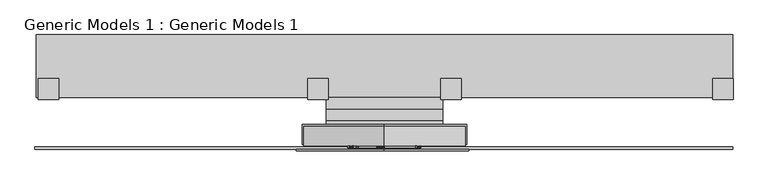
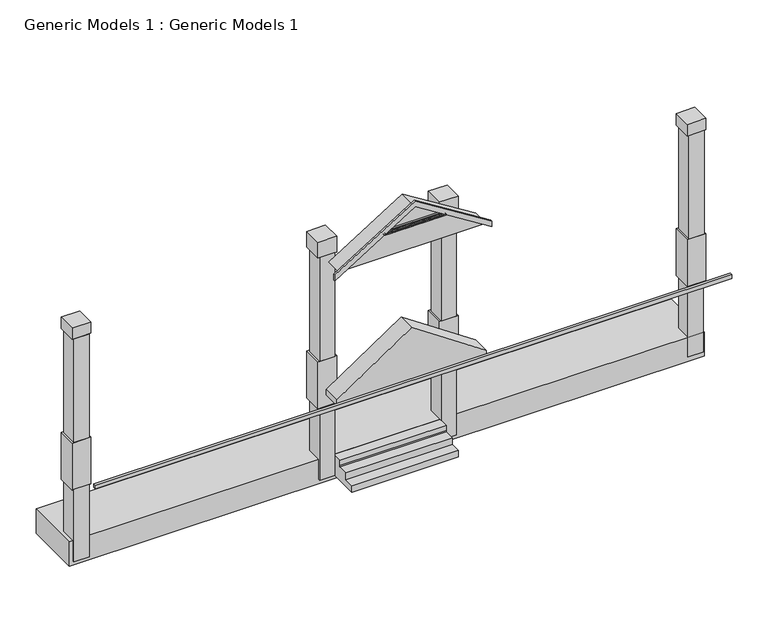
"""IFC4 building model written with IfcOpenShell, lengths in millimetres: proxy geometry, Generic Models 1 : Generic Models 1."""

from ifc_helpers import new_model, si_unit, point, frame, frame_2d, origin, place, context, project, spatial, polyline, circle_curve, trimmed, segment, composite_curve, outline, extrude, source, transform, mapped, element, save


def generic_models_1_generic_models_1_befc9ee0(model_context):
    return source(origin(), model_context, "Body", "SweptSolid", [
        extrude(outline(composite_curve([segment(trimmed(circle_curve(frame_2d((7938.0752919, -1466.3553383)), 19.05), [point((7948.1702538, -1450.2000221))], [point((7927.9803299, -1482.5106546))], False, "CARTESIAN"), True, "CONTINUOUS"), segment(trimmed(circle_curve(frame_2d((7938.0752919, -1466.3553383)), 19.05), [point((7927.9803299, -1482.5106546))], [point((7948.1702538, -1450.2000221))], False, "CARTESIAN"), True, "CONTINUOUS")], self_intersect=False)), frame((0.0, -10111.4037218, 0.0), z_axis=(0.0, 1.0, 0.0), x_axis=(0.0, 0.0, 1.0)), (0.0, 0.0, 1.0), 50.8),
        extrude(outline(composite_curve([segment(trimmed(circle_curve(frame_2d((7938.0752919, -1383.8053383)), 19.05), [point((7948.1702538, -1367.6500221))], [point((7927.9803299, -1399.9606546))], False, "CARTESIAN"), True, "CONTINUOUS"), segment(trimmed(circle_curve(frame_2d((7938.0752919, -1383.8053383)), 19.05), [point((7927.9803299, -1399.9606546))], [point((7948.1702538, -1367.6500221))], False, "CARTESIAN"), True, "CONTINUOUS")], self_intersect=False)), frame((0.0, -10111.4037218, 0.0), z_axis=(0.0, 1.0, 0.0), x_axis=(0.0, 0.0, 1.0)), (0.0, 0.0, 1.0), 50.8),
        extrude(outline(composite_curve([segment(trimmed(circle_curve(frame_2d((7938.0752919, -1326.6553383)), 19.05), [point((7948.1702538, -1310.5000221))], [point((7927.9803299, -1342.8106546))], False, "CARTESIAN"), True, "CONTINUOUS"), segment(trimmed(circle_curve(frame_2d((7938.0752919, -1326.6553383)), 19.05), [point((7927.9803299, -1342.8106546))], [point((7948.1702538, -1310.5000221))], False, "CARTESIAN"), True, "CONTINUOUS")], self_intersect=False)), frame((0.0, -10111.4037218, 0.0), z_axis=(0.0, 1.0, 0.0), x_axis=(0.0, 0.0, 1.0)), (0.0, 0.0, 1.0), 50.8),
        extrude(outline(composite_curve([segment(trimmed(circle_curve(frame_2d((7938.0752919, -1275.8553383)), 19.05), [point((7948.1702538, -1259.7000221))], [point((7927.9803299, -1292.0106546))], False, "CARTESIAN"), True, "CONTINUOUS"), segment(trimmed(circle_curve(frame_2d((7938.0752919, -1275.8553383)), 19.05), [point((7927.9803299, -1292.0106546))], [point((7948.1702538, -1259.7000221))], False, "CARTESIAN"), True, "CONTINUOUS")], self_intersect=False)), frame((0.0, -10111.4037218, 0.0), z_axis=(0.0, 1.0, 0.0), x_axis=(0.0, 0.0, 1.0)), (0.0, 0.0, 1.0), 50.8),
        extrude(outline(composite_curve([segment(trimmed(circle_curve(frame_2d((7938.0752919, -1225.0553383)), 19.05), [point((7948.1702538, -1208.9000221))], [point((7927.9803299, -1241.2106546))], False, "CARTESIAN"), True, "CONTINUOUS"), segment(trimmed(circle_curve(frame_2d((7938.0752919, -1225.0553383)), 19.05), [point((7927.9803299, -1241.2106546))], [point((7948.1702538, -1208.9000221))], False, "CARTESIAN"), True, "CONTINUOUS")], self_intersect=False)), frame((0.0, -10111.4037218, 0.0), z_axis=(0.0, 1.0, 0.0), x_axis=(0.0, 0.0, 1.0)), (0.0, 0.0, 1.0), 50.8),
        extrude(outline(composite_curve([segment(trimmed(circle_curve(frame_2d((7938.0752919, -1180.6053383)), 19.05), [point((7948.1702538, -1164.4500221))], [point((7927.9803299, -1196.7606546))], False, "CARTESIAN"), True, "CONTINUOUS"), segment(trimmed(circle_curve(frame_2d((7938.0752919, -1180.6053383)), 19.05), [point((7927.9803299, -1196.7606546))], [point((7948.1702538, -1164.4500221))], False, "CARTESIAN"), True, "CONTINUOUS")], self_intersect=False)), frame((0.0, -10111.4037218, 0.0), z_axis=(0.0, 1.0, 0.0), x_axis=(0.0, 0.0, 1.0)), (0.0, 0.0, 1.0), 50.8),
        extrude(outline(composite_curve([segment(trimmed(circle_curve(frame_2d((7938.0752919, -1138.428657)), 19.05), [point((7948.1702538, -1122.2733408))], [point((7927.9803299, -1154.5839732))], False, "CARTESIAN"), True, "CONTINUOUS"), segment(trimmed(circle_curve(frame_2d((7938.0752919, -1138.428657)), 19.05), [point((7927.9803299, -1154.5839732))], [point((7948.1702538, -1122.2733408))], False, "CARTESIAN"), True, "CONTINUOUS")], self_intersect=False)), frame((0.0, -10111.4037218, 0.0), z_axis=(0.0, 1.0, 0.0), x_axis=(0.0, 0.0, 1.0)), (0.0, 0.0, 1.0), 50.8),
        extrude(outline(composite_curve([segment(trimmed(circle_curve(frame_2d((7938.0752919, -1097.6641631)), 19.05), [point((7948.1702538, -1081.5088469))], [point((7927.9803299, -1113.8194794))], False, "CARTESIAN"), True, "CONTINUOUS"), segment(trimmed(circle_curve(frame_2d((7938.0752919, -1097.6641631)), 19.05), [point((7927.9803299, -1113.8194794))], [point((7948.1702538, -1081.5088469))], False, "CARTESIAN"), True, "CONTINUOUS")], self_intersect=False)), frame((0.0, -10111.4037218, 0.0), z_axis=(0.0, 1.0, 0.0), x_axis=(0.0, 0.0, 1.0)), (0.0, 0.0, 1.0), 50.8),
        extrude(outline(composite_curve([segment(trimmed(circle_curve(frame_2d((7938.0752919, -1056.7520685)), 19.05), [point((7948.1702538, -1040.5967523))], [point((7927.9803299, -1072.9073848))], False, "CARTESIAN"), True, "CONTINUOUS"), segment(trimmed(circle_curve(frame_2d((7938.0752919, -1056.7520685)), 19.05), [point((7927.9803299, -1072.9073848))], [point((7948.1702538, -1040.5967523))], False, "CARTESIAN"), True, "CONTINUOUS")], self_intersect=False)), frame((0.0, -10111.4037218, 0.0), z_axis=(0.0, 1.0, 0.0), x_axis=(0.0, 0.0, 1.0)), (0.0, 0.0, 1.0), 50.8),
        extrude(outline(composite_curve([segment(trimmed(circle_curve(frame_2d((7938.0752919, -1016.280255)), 19.05), [point((7948.1702538, -1000.1249387))], [point((7927.9803299, -1032.4355712))], False, "CARTESIAN"), True, "CONTINUOUS"), segment(trimmed(circle_curve(frame_2d((7938.0752919, -1016.280255)), 19.05), [point((7927.9803299, -1032.4355712))], [point((7948.1702538, -1000.1249387))], False, "CARTESIAN"), True, "CONTINUOUS")], self_intersect=False)), frame((0.0, -10111.4037218, 0.0), z_axis=(0.0, 1.0, 0.0), x_axis=(0.0, 0.0, 1.0)), (0.0, 0.0, 1.0), 50.8),
        extrude(outline(composite_curve([segment(trimmed(circle_curve(frame_2d((7938.0752919, -976.8863285)), 19.05), [point((7948.1702538, -960.7310122))], [point((7927.9803299, -993.0416447))], False, "CARTESIAN"), True, "CONTINUOUS"), segment(trimmed(circle_curve(frame_2d((7938.0752919, -976.8863285)), 19.05), [point((7927.9803299, -993.0416447))], [point((7948.1702538, -960.7310122))], False, "CARTESIAN"), True, "CONTINUOUS")], self_intersect=False)), frame((0.0, -10111.4037218, 0.0), z_axis=(0.0, 1.0, 0.0), x_axis=(0.0, 0.0, 1.0)), (0.0, 0.0, 1.0), 50.8),
        extrude(outline(composite_curve([segment(trimmed(circle_curve(frame_2d((7938.0752919, -936.520986)), 19.05), [point((7948.1702538, -920.3656697))], [point((7927.9803299, -952.6763022))], False, "CARTESIAN"), True, "CONTINUOUS"), segment(trimmed(circle_curve(frame_2d((7938.0752919, -936.520986)), 19.05), [point((7927.9803299, -952.6763022))], [point((7948.1702538, -920.3656697))], False, "CARTESIAN"), True, "CONTINUOUS")], self_intersect=False)), frame((0.0, -10111.4037218, 0.0), z_axis=(0.0, 1.0, 0.0), x_axis=(0.0, 0.0, 1.0)), (0.0, 0.0, 1.0), 50.8),
        extrude(outline(composite_curve([segment(trimmed(circle_curve(frame_2d((7938.0752919, -896.4770473)), 19.05), [point((7948.1702538, -880.3217311))], [point((7927.9803299, -912.6323636))], False, "CARTESIAN"), True, "CONTINUOUS"), segment(trimmed(circle_curve(frame_2d((7938.0752919, -896.4770473)), 19.05), [point((7927.9803299, -912.6323636))], [point((7948.1702538, -880.3217311))], False, "CARTESIAN"), True, "CONTINUOUS")], self_intersect=False)), frame((0.0, -10111.4037218, 0.0), z_axis=(0.0, 1.0, 0.0), x_axis=(0.0, 0.0, 1.0)), (0.0, 0.0, 1.0), 50.8),
        extrude(outline(composite_curve([segment(trimmed(circle_curve(frame_2d((7938.0752919, -855.7356566)), 19.05), [point((7948.1702538, -839.5803404))], [point((7927.9803299, -871.8909729))], False, "CARTESIAN"), True, "CONTINUOUS"), segment(trimmed(circle_curve(frame_2d((7938.0752919, -855.7356566)), 19.05), [point((7927.9803299, -871.8909729))], [point((7948.1702538, -839.5803404))], False, "CARTESIAN"), True, "CONTINUOUS")], self_intersect=False)), frame((0.0, -10111.4037218, 0.0), z_axis=(0.0, 1.0, 0.0), x_axis=(0.0, 0.0, 1.0)), (0.0, 0.0, 1.0), 50.8),
        extrude(outline(composite_curve([segment(trimmed(circle_curve(frame_2d((7938.0752919, -814.8009363)), 19.05), [point((7948.1702538, -798.64562))], [point((7927.9803299, -830.9562525))], False, "CARTESIAN"), True, "CONTINUOUS"), segment(trimmed(circle_curve(frame_2d((7938.0752919, -814.8009363)), 19.05), [point((7927.9803299, -830.9562525))], [point((7948.1702538, -798.64562))], False, "CARTESIAN"), True, "CONTINUOUS")], self_intersect=False)), frame((0.0, -10111.4037218, 0.0), z_axis=(0.0, 1.0, 0.0), x_axis=(0.0, 0.0, 1.0)), (0.0, 0.0, 1.0), 50.8),
        extrude(outline(composite_curve([segment(trimmed(circle_curve(frame_2d((7938.0752919, -773.5784958)), 19.05), [point((7948.1702538, -757.4231795))], [point((7927.9803299, -789.733812))], False, "CARTESIAN"), True, "CONTINUOUS"), segment(trimmed(circle_curve(frame_2d((7938.0752919, -773.5784958)), 19.05), [point((7927.9803299, -789.733812))], [point((7948.1702538, -757.4231795))], False, "CARTESIAN"), True, "CONTINUOUS")], self_intersect=False)), frame((0.0, -10111.4037218, 0.0), z_axis=(0.0, 1.0, 0.0), x_axis=(0.0, 0.0, 1.0)), (0.0, 0.0, 1.0), 50.8),
        extrude(outline(composite_curve([segment(trimmed(circle_curve(frame_2d((7938.0752919, -733.1581785)), 19.05), [point((7948.1702538, -717.0028623))], [point((7927.9803299, -749.3134947))], False, "CARTESIAN"), True, "CONTINUOUS"), segment(trimmed(circle_curve(frame_2d((7938.0752919, -733.1581785)), 19.05), [point((7927.9803299, -749.3134947))], [point((7948.1702538, -717.0028623))], False, "CARTESIAN"), True, "CONTINUOUS")], self_intersect=False)), frame((0.0, -10111.4037218, 0.0), z_axis=(0.0, 1.0, 0.0), x_axis=(0.0, 0.0, 1.0)), (0.0, 0.0, 1.0), 50.8),
        extrude(outline(composite_curve([segment(trimmed(circle_curve(frame_2d((7938.0752919, -692.1370435)), 19.05), [point((7948.1702538, -675.9817273))], [point((7927.9803299, -708.2923598))], False, "CARTESIAN"), True, "CONTINUOUS"), segment(trimmed(circle_curve(frame_2d((7938.0752919, -692.1370435)), 19.05), [point((7927.9803299, -708.2923598))], [point((7948.1702538, -675.9817273))], False, "CARTESIAN"), True, "CONTINUOUS")], self_intersect=False)), frame((0.0, -10111.4037218, 0.0), z_axis=(0.0, 1.0, 0.0), x_axis=(0.0, 0.0, 1.0)), (0.0, 0.0, 1.0), 50.8),
        extrude(outline(composite_curve([segment(trimmed(circle_curve(frame_2d((7938.0752919, -652.3790926)), 19.05), [point((7948.1702538, -636.2237763))], [point((7927.9803299, -668.5344088))], False, "CARTESIAN"), True, "CONTINUOUS"), segment(trimmed(circle_curve(frame_2d((7938.0752919, -652.3790926)), 19.05), [point((7927.9803299, -668.5344088))], [point((7948.1702538, -636.2237763))], False, "CARTESIAN"), True, "CONTINUOUS")], self_intersect=False)), frame((0.0, -10111.4037218, 0.0), z_axis=(0.0, 1.0, 0.0), x_axis=(0.0, 0.0, 1.0)), (0.0, 0.0, 1.0), 50.8),
        extrude(outline(composite_curve([segment(trimmed(circle_curve(frame_2d((7938.0752919, -612.5240225)), 19.05), [point((7948.1702538, -596.3687063))], [point((7927.9803299, -628.6793387))], False, "CARTESIAN"), True, "CONTINUOUS"), segment(trimmed(circle_curve(frame_2d((7938.0752919, -612.5240225)), 19.05), [point((7927.9803299, -628.6793387))], [point((7948.1702538, -596.3687063))], False, "CARTESIAN"), True, "CONTINUOUS")], self_intersect=False)), frame((0.0, -10111.4037218, 0.0), z_axis=(0.0, 1.0, 0.0), x_axis=(0.0, 0.0, 1.0)), (0.0, 0.0, 1.0), 50.8),
        extrude(outline(composite_curve([segment(trimmed(circle_curve(frame_2d((7938.0752919, -572.3055332)), 19.05), [point((7948.1702538, -556.150217))], [point((7927.9803299, -588.4608494))], False, "CARTESIAN"), True, "CONTINUOUS"), segment(trimmed(circle_curve(frame_2d((7938.0752919, -572.3055332)), 19.05), [point((7927.9803299, -588.4608494))], [point((7948.1702538, -556.150217))], False, "CARTESIAN"), True, "CONTINUOUS")], self_intersect=False)), frame((0.0, -10111.4037218, 0.0), z_axis=(0.0, 1.0, 0.0), x_axis=(0.0, 0.0, 1.0)), (0.0, 0.0, 1.0), 50.8),
        extrude(outline(composite_curve([segment(trimmed(circle_curve(frame_2d((7938.0752919, -531.6918396)), 19.05), [point((7948.1702538, -515.5365234))], [point((7927.9803299, -547.8471558))], False, "CARTESIAN"), True, "CONTINUOUS"), segment(trimmed(circle_curve(frame_2d((7938.0752919, -531.6918396)), 19.05), [point((7927.9803299, -547.8471558))], [point((7948.1702538, -515.5365234))], False, "CARTESIAN"), True, "CONTINUOUS")], self_intersect=False)), frame((0.0, -10111.4037218, 0.0), z_axis=(0.0, 1.0, 0.0), x_axis=(0.0, 0.0, 1.0)), (0.0, 0.0, 1.0), 50.8),
        extrude(outline(composite_curve([segment(trimmed(circle_curve(frame_2d((7938.0752919, -491.0257527)), 19.05), [point((7948.1702538, -474.8704364))], [point((7927.9803299, -507.1810689))], False, "CARTESIAN"), True, "CONTINUOUS"), segment(trimmed(circle_curve(frame_2d((7938.0752919, -491.0257527)), 19.05), [point((7927.9803299, -507.1810689))], [point((7948.1702538, -474.8704364))], False, "CARTESIAN"), True, "CONTINUOUS")], self_intersect=False)), frame((0.0, -10111.4037218, 0.0), z_axis=(0.0, 1.0, 0.0), x_axis=(0.0, 0.0, 1.0)), (0.0, 0.0, 1.0), 50.8),
        extrude(outline(composite_curve([segment(trimmed(circle_curve(frame_2d((7938.0752919, -450.4847688)), 19.05), [point((7948.1702538, -434.3294526))], [point((7927.9803299, -466.6400851))], False, "CARTESIAN"), True, "CONTINUOUS"), segment(trimmed(circle_curve(frame_2d((7938.0752919, -450.4847688)), 19.05), [point((7927.9803299, -466.6400851))], [point((7948.1702538, -434.3294526))], False, "CARTESIAN"), True, "CONTINUOUS")], self_intersect=False)), frame((0.0, -10111.4037218, 0.0), z_axis=(0.0, 1.0, 0.0), x_axis=(0.0, 0.0, 1.0)), (0.0, 0.0, 1.0), 50.8),
        extrude(outline(composite_curve([segment(trimmed(circle_curve(frame_2d((7938.0752919, -410.3323364)), 19.05), [point((7948.1702538, -394.1770202))], [point((7927.9803299, -426.4876527))], False, "CARTESIAN"), True, "CONTINUOUS"), segment(trimmed(circle_curve(frame_2d((7938.0752919, -410.3323364)), 19.05), [point((7927.9803299, -426.4876527))], [point((7948.1702538, -394.1770202))], False, "CARTESIAN"), True, "CONTINUOUS")], self_intersect=False)), frame((0.0, -10111.4037218, 0.0), z_axis=(0.0, 1.0, 0.0), x_axis=(0.0, 0.0, 1.0)), (0.0, 0.0, 1.0), 50.8),
        extrude(outline(composite_curve([segment(trimmed(circle_curve(frame_2d((7938.0752919, -368.9951349)), 19.05), [point((7948.1702538, -352.8398187))], [point((7927.9803299, -385.1504511))], False, "CARTESIAN"), True, "CONTINUOUS"), segment(trimmed(circle_curve(frame_2d((7938.0752919, -368.9951349)), 19.05), [point((7927.9803299, -385.1504511))], [point((7948.1702538, -352.8398187))], False, "CARTESIAN"), True, "CONTINUOUS")], self_intersect=False)), frame((0.0, -10111.4037218, 0.0), z_axis=(0.0, 1.0, 0.0), x_axis=(0.0, 0.0, 1.0)), (0.0, 0.0, 1.0), 50.8),
        extrude(outline(composite_curve([segment(trimmed(circle_curve(frame_2d((7938.0752919, -327.345884)), 19.05), [point((7948.1702538, -311.1905678))], [point((7927.9803299, -343.5012002))], False, "CARTESIAN"), True, "CONTINUOUS"), segment(trimmed(circle_curve(frame_2d((7938.0752919, -327.345884)), 19.05), [point((7927.9803299, -343.5012002))], [point((7948.1702538, -311.1905678))], False, "CARTESIAN"), True, "CONTINUOUS")], self_intersect=False)), frame((0.0, -10111.4037218, 0.0), z_axis=(0.0, 1.0, 0.0), x_axis=(0.0, 0.0, 1.0)), (0.0, 0.0, 1.0), 50.8),
        extrude(outline(composite_curve([segment(trimmed(circle_curve(frame_2d((7938.0752919, -287.0633181)), 19.05), [point((7948.1702538, -270.9080019))], [point((7927.9803299, -303.2186343))], False, "CARTESIAN"), True, "CONTINUOUS"), segment(trimmed(circle_curve(frame_2d((7938.0752919, -287.0633181)), 19.05), [point((7927.9803299, -303.2186343))], [point((7948.1702538, -270.9080019))], False, "CARTESIAN"), True, "CONTINUOUS")], self_intersect=False)), frame((0.0, -10111.4037218, 0.0), z_axis=(0.0, 1.0, 0.0), x_axis=(0.0, 0.0, 1.0)), (0.0, 0.0, 1.0), 50.8),
        extrude(outline(composite_curve([segment(trimmed(circle_curve(frame_2d((7938.0752919, -247.7040917)), 19.05), [point((7948.1702538, -231.5487755))], [point((7927.9803299, -263.8594079))], False, "CARTESIAN"), True, "CONTINUOUS"), segment(trimmed(circle_curve(frame_2d((7938.0752919, -247.7040917)), 19.05), [point((7927.9803299, -263.8594079))], [point((7948.1702538, -231.5487755))], False, "CARTESIAN"), True, "CONTINUOUS")], self_intersect=False)), frame((0.0, -10111.4037218, 0.0), z_axis=(0.0, 1.0, 0.0), x_axis=(0.0, 0.0, 1.0)), (0.0, 0.0, 1.0), 50.8),
        extrude(outline(composite_curve([segment(trimmed(circle_curve(frame_2d((7938.0752919, -208.2693222)), 19.05), [point((7948.1702538, -192.114006))], [point((7927.9803299, -224.4246384))], False, "CARTESIAN"), True, "CONTINUOUS"), segment(trimmed(circle_curve(frame_2d((7938.0752919, -208.2693222)), 19.05), [point((7927.9803299, -224.4246384))], [point((7948.1702538, -192.114006))], False, "CARTESIAN"), True, "CONTINUOUS")], self_intersect=False)), frame((0.0, -10111.4037218, 0.0), z_axis=(0.0, 1.0, 0.0), x_axis=(0.0, 0.0, 1.0)), (0.0, 0.0, 1.0), 50.8),
        extrude(outline(composite_curve([segment(trimmed(circle_curve(frame_2d((7938.0752919, -168.7855995)), 19.05), [point((7948.1702538, -152.6302833))], [point((7927.9803299, -184.9409158))], False, "CARTESIAN"), True, "CONTINUOUS"), segment(trimmed(circle_curve(frame_2d((7938.0752919, -168.7855995)), 19.05), [point((7927.9803299, -184.9409158))], [point((7948.1702538, -152.6302833))], False, "CARTESIAN"), True, "CONTINUOUS")], self_intersect=False)), frame((0.0, -10111.4037218, 0.0), z_axis=(0.0, 1.0, 0.0), x_axis=(0.0, 0.0, 1.0)), (0.0, 0.0, 1.0), 50.8),
        extrude(outline(composite_curve([segment(trimmed(circle_curve(frame_2d((7938.0752919, -129.2343587)), 19.05), [point((7948.1702538, -113.0790425))], [point((7927.9803299, -145.389675))], False, "CARTESIAN"), True, "CONTINUOUS"), segment(trimmed(circle_curve(frame_2d((7938.0752919, -129.2343587)), 19.05), [point((7927.9803299, -145.389675))], [point((7948.1702538, -113.0790425))], False, "CARTESIAN"), True, "CONTINUOUS")], self_intersect=False)), frame((0.0, -10111.4037218, 0.0), z_axis=(0.0, 1.0, 0.0), x_axis=(0.0, 0.0, 1.0)), (0.0, 0.0, 1.0), 50.8),
        extrude(outline(composite_curve([segment(trimmed(circle_curve(frame_2d((7938.0752919, -85.7359946)), 19.05), [point((7948.1702538, -69.5806784))], [point((7927.9803299, -101.8913108))], False, "CARTESIAN"), True, "CONTINUOUS"), segment(trimmed(circle_curve(frame_2d((7938.0752919, -85.7359946)), 19.05), [point((7927.9803299, -101.8913108))], [point((7948.1702538, -69.5806784))], False, "CARTESIAN"), True, "CONTINUOUS")], self_intersect=False)), frame((0.0, -10111.4037218, 0.0), z_axis=(0.0, 1.0, 0.0), x_axis=(0.0, 0.0, 1.0)), (0.0, 0.0, 1.0), 50.8),
        extrude(outline(composite_curve([segment(trimmed(circle_curve(frame_2d((7938.0752919, -45.637188)), 19.05), [point((7948.1702538, -29.4818718))], [point((7927.9803299, -61.7925043))], False, "CARTESIAN"), True, "CONTINUOUS"), segment(trimmed(circle_curve(frame_2d((7938.0752919, -45.637188)), 19.05), [point((7927.9803299, -61.7925043))], [point((7948.1702538, -29.4818718))], False, "CARTESIAN"), True, "CONTINUOUS")], self_intersect=False)), frame((0.0, -10111.4037218, 0.0), z_axis=(0.0, 1.0, 0.0), x_axis=(0.0, 0.0, 1.0)), (0.0, 0.0, 1.0), 50.8),
        extrude(outline(composite_curve([segment(trimmed(circle_curve(frame_2d((7938.0752919, -5.8865584)), 19.05), [point((7948.1702538, 10.2687578))], [point((7927.9803299, -22.0418747))], False, "CARTESIAN"), True, "CONTINUOUS"), segment(trimmed(circle_curve(frame_2d((7938.0752919, -5.8865584)), 19.05), [point((7927.9803299, -22.0418747))], [point((7948.1702538, 10.2687578))], False, "CARTESIAN"), True, "CONTINUOUS")], self_intersect=False)), frame((0.0, -10111.4037218, 0.0), z_axis=(0.0, 1.0, 0.0), x_axis=(0.0, 0.0, 1.0)), (0.0, 0.0, 1.0), 50.8),
        extrude(outline(composite_curve([segment(trimmed(circle_curve(frame_2d((7938.0752919, 33.7092744)), 19.05), [point((7948.1702538, 49.8645907))], [point((7927.9803299, 17.5539582))], False, "CARTESIAN"), True, "CONTINUOUS"), segment(trimmed(circle_curve(frame_2d((7938.0752919, 33.7092744)), 19.05), [point((7927.9803299, 17.5539582))], [point((7948.1702538, 49.8645907))], False, "CARTESIAN"), True, "CONTINUOUS")], self_intersect=False)), frame((0.0, -10111.4037218, 0.0), z_axis=(0.0, 1.0, 0.0), x_axis=(0.0, 0.0, 1.0)), (0.0, 0.0, 1.0), 50.8),
        extrude(outline(composite_curve([segment(trimmed(circle_curve(frame_2d((7938.0752919, 73.2770088)), 19.05), [point((7948.1702538, 89.432325))], [point((7927.9803299, 57.1216925))], False, "CARTESIAN"), True, "CONTINUOUS"), segment(trimmed(circle_curve(frame_2d((7938.0752919, 73.2770088)), 19.05), [point((7927.9803299, 57.1216925))], [point((7948.1702538, 89.432325))], False, "CARTESIAN"), True, "CONTINUOUS")], self_intersect=False)), frame((0.0, -10111.4037218, 0.0), z_axis=(0.0, 1.0, 0.0), x_axis=(0.0, 0.0, 1.0)), (0.0, 0.0, 1.0), 50.8),
        extrude(outline(composite_curve([segment(trimmed(circle_curve(frame_2d((7938.0752919, 112.7643199)), 19.05), [point((7948.1702538, 128.9196362))], [point((7927.9803299, 96.6090037))], False, "CARTESIAN"), True, "CONTINUOUS"), segment(trimmed(circle_curve(frame_2d((7938.0752919, 112.7643199)), 19.05), [point((7927.9803299, 96.6090037))], [point((7948.1702538, 128.9196362))], False, "CARTESIAN"), True, "CONTINUOUS")], self_intersect=False)), frame((0.0, -10111.4037218, 0.0), z_axis=(0.0, 1.0, 0.0), x_axis=(0.0, 0.0, 1.0)), (0.0, 0.0, 1.0), 50.8),
        extrude(outline(composite_curve([segment(trimmed(circle_curve(frame_2d((7938.0752919, 152.2302668)), 19.05), [point((7948.1702538, 168.385583))], [point((7927.9803299, 136.0749506))], False, "CARTESIAN"), True, "CONTINUOUS"), segment(trimmed(circle_curve(frame_2d((7938.0752919, 152.2302668)), 19.05), [point((7927.9803299, 136.0749506))], [point((7948.1702538, 168.385583))], False, "CARTESIAN"), True, "CONTINUOUS")], self_intersect=False)), frame((0.0, -10111.4037218, 0.0), z_axis=(0.0, 1.0, 0.0), x_axis=(0.0, 0.0, 1.0)), (0.0, 0.0, 1.0), 50.8),
        extrude(outline(composite_curve([segment(trimmed(circle_curve(frame_2d((7938.0752919, 192.2239734)), 19.05), [point((7948.1702538, 208.3792897))], [point((7927.9803299, 176.0686572))], False, "CARTESIAN"), True, "CONTINUOUS"), segment(trimmed(circle_curve(frame_2d((7938.0752919, 192.2239734)), 19.05), [point((7927.9803299, 176.0686572))], [point((7948.1702538, 208.3792897))], False, "CARTESIAN"), True, "CONTINUOUS")], self_intersect=False)), frame((0.0, -10111.4037218, 0.0), z_axis=(0.0, 1.0, 0.0), x_axis=(0.0, 0.0, 1.0)), (0.0, 0.0, 1.0), 50.8),
        extrude(outline(composite_curve([segment(trimmed(circle_curve(frame_2d((7938.0752919, 232.0701465)), 19.05), [point((7948.1702538, 248.2254628))], [point((7927.9803299, 215.9148303))], False, "CARTESIAN"), True, "CONTINUOUS"), segment(trimmed(circle_curve(frame_2d((7938.0752919, 232.0701465)), 19.05), [point((7927.9803299, 215.9148303))], [point((7948.1702538, 248.2254628))], False, "CARTESIAN"), True, "CONTINUOUS")], self_intersect=False)), frame((0.0, -10111.4037218, 0.0), z_axis=(0.0, 1.0, 0.0), x_axis=(0.0, 0.0, 1.0)), (0.0, 0.0, 1.0), 50.8),
        extrude(outline(composite_curve([segment(trimmed(circle_curve(frame_2d((7938.0752919, 271.3681213)), 19.05), [point((7948.1702538, 287.5234376))], [point((7927.9803299, 255.2128051))], False, "CARTESIAN"), True, "CONTINUOUS"), segment(trimmed(circle_curve(frame_2d((7938.0752919, 271.3681213)), 19.05), [point((7927.9803299, 255.2128051))], [point((7948.1702538, 287.5234376))], False, "CARTESIAN"), True, "CONTINUOUS")], self_intersect=False)), frame((0.0, -10111.4037218, 0.0), z_axis=(0.0, 1.0, 0.0), x_axis=(0.0, 0.0, 1.0)), (0.0, 0.0, 1.0), 50.8),
        extrude(outline(composite_curve([segment(trimmed(circle_curve(frame_2d((7938.0752919, 312.0288686)), 19.05), [point((7948.1702538, 328.1841848))], [point((7927.9803299, 295.8735524))], False, "CARTESIAN"), True, "CONTINUOUS"), segment(trimmed(circle_curve(frame_2d((7938.0752919, 312.0288686)), 19.05), [point((7927.9803299, 295.8735524))], [point((7948.1702538, 328.1841848))], False, "CARTESIAN"), True, "CONTINUOUS")], self_intersect=False)), frame((0.0, -10111.4037218, 0.0), z_axis=(0.0, 1.0, 0.0), x_axis=(0.0, 0.0, 1.0)), (0.0, 0.0, 1.0), 50.8),
        extrude(outline(composite_curve([segment(trimmed(circle_curve(frame_2d((7938.0752919, 354.3706857)), 19.05), [point((7948.1702538, 370.5260019))], [point((7927.9803299, 338.2153695))], False, "CARTESIAN"), True, "CONTINUOUS"), segment(trimmed(circle_curve(frame_2d((7938.0752919, 354.3706857)), 19.05), [point((7927.9803299, 338.2153695))], [point((7948.1702538, 370.5260019))], False, "CARTESIAN"), True, "CONTINUOUS")], self_intersect=False)), frame((0.0, -10111.4037218, 0.0), z_axis=(0.0, 1.0, 0.0), x_axis=(0.0, 0.0, 1.0)), (0.0, 0.0, 1.0), 50.8),
        extrude(outline(composite_curve([segment(trimmed(circle_curve(frame_2d((7938.0752919, 394.6506107)), 19.05), [point((7948.1702538, 410.8059269))], [point((7927.9803299, 378.4952944))], False, "CARTESIAN"), True, "CONTINUOUS"), segment(trimmed(circle_curve(frame_2d((7938.0752919, 394.6506107)), 19.05), [point((7927.9803299, 378.4952944))], [point((7948.1702538, 410.8059269))], False, "CARTESIAN"), True, "CONTINUOUS")], self_intersect=False)), frame((0.0, -10111.4037218, 0.0), z_axis=(0.0, 1.0, 0.0), x_axis=(0.0, 0.0, 1.0)), (0.0, 0.0, 1.0), 50.8),
        extrude(outline(composite_curve([segment(trimmed(circle_curve(frame_2d((7938.0752919, 434.6778162)), 19.05), [point((7948.1702538, 450.8331325))], [point((7927.9803299, 418.5225))], False, "CARTESIAN"), True, "CONTINUOUS"), segment(trimmed(circle_curve(frame_2d((7938.0752919, 434.6778162)), 19.05), [point((7927.9803299, 418.5225))], [point((7948.1702538, 450.8331325))], False, "CARTESIAN"), True, "CONTINUOUS")], self_intersect=False)), frame((0.0, -10111.4037218, 0.0), z_axis=(0.0, 1.0, 0.0), x_axis=(0.0, 0.0, 1.0)), (0.0, 0.0, 1.0), 50.8),
        extrude(outline(composite_curve([segment(trimmed(circle_curve(frame_2d((7938.0752919, -1424.0920784)), 19.05), [point((7948.1702538, -1407.9367621))], [point((7927.9803299, -1440.2473946))], False, "CARTESIAN"), True, "CONTINUOUS"), segment(trimmed(circle_curve(frame_2d((7938.0752919, -1424.0920784)), 19.05), [point((7927.9803299, -1440.2473946))], [point((7948.1702538, -1407.9367621))], False, "CARTESIAN"), True, "CONTINUOUS")], self_intersect=False)), frame((0.0, -10111.4037218, 0.0), z_axis=(0.0, 1.0, 0.0), x_axis=(0.0, 0.0, 1.0)), (0.0, 0.0, 1.0), 50.8),
        extrude(outline(polyline([(8047.4435422, 304.748165), (8047.4435422, -1329.0322968), (8021.2835928, -1370.896967), (8021.2835928, 346.6128352), (8047.4435422, 304.748165)])), frame((0.0, -10111.4037218, 0.0), z_axis=(0.0, 1.0, 0.0), x_axis=(0.0, 0.0, 1.0)), (0.0, 0.0, 1.0), 50.8),
        extrude(outline(polyline([(8557.8932113, -512.1420659), (7216.244263, -2659.2292037), (7216.244263, 1634.9450719), (8557.8932113, -512.1420659)])), frame((0.0, -10060.6037218, 0.0), z_axis=(0.0, 1.0, 0.0), x_axis=(0.0, 0.0, 1.0)), (0.0, 0.0, 1.0), 515.4980224),
        extrude(outline(polyline([(8737.6, -512.1420659), (7270.465525, -2860.0480249), (7090.7587364, -2860.0480249), (8557.8932113, -512.1420659), (7158.0584829, 1728.0617849), (7337.7652716, 1728.0617849), (8737.6, -512.1420659)])), frame((0.0, -10199.2878342, 0.0), z_axis=(0.0, 1.0, 0.0), x_axis=(0.0, 0.0, 1.0)), (0.0, 0.0, 1.0), 50.8),
        extrude(outline(polyline([(8746.1579341, -10156.9067839), (-9809.6634433, -10156.9067839), (-9809.6634433, -10080.7067839), (8746.1579341, -10080.7067839), (8746.1579341, -10156.9067839)])), frame((0.0, 0.0, 3085.2974515), z_axis=(0.0, 0.0, 1.0), x_axis=(1.0, 0.0, 0.0)), (0.0, 0.0, 1.0), 116.0225688),
        extrude(outline(polyline([(4724.4, -512.1420659), (3252.1200204, -2694.8868984), (3085.2974515, -2694.8868984), (3085.2974515, 1670.6027667), (3252.1200204, 1670.6027667), (4724.4, -512.1420659)])), frame((0.0, -10022.4331537, 0.0), z_axis=(0.0, 1.0, 0.0), x_axis=(0.0, 0.0, 1.0)), (0.0, 0.0, 1.0), 534.7930857),
        extrude(outline(polyline([(8758.8579341, -8825.9902135), (8212.7579341, -8825.9902135), (8212.7579341, -8267.1902135), (8758.8579341, -8267.1902135), (8758.8579341, -8825.9902135)])), frame((0.0, 0.0, 6858.0), z_axis=(0.0, 0.0, 1.0), x_axis=(1.0, 0.0, 0.0)), (0.0, 0.0, 1.0), 352.8293402),
        extrude(outline(polyline([(8708.0579341, -8825.9902135), (8263.5579341, -8825.9902135), (8263.5579341, -8317.9902135), (8708.0579341, -8317.9902135), (8708.0579341, -8825.9902135)])), frame((0.0, 0.0, 3657.6), z_axis=(0.0, 0.0, 1.0), x_axis=(1.0, 0.0, 0.0)), (0.0, 0.0, 1.0), 3200.4),
        extrude(outline(polyline([(8758.8579341, -8825.9902135), (8212.7579341, -8825.9902135), (8212.7579341, -8267.1902135), (8758.8579341, -8267.1902135), (8758.8579341, -8825.9902135)])), frame((0.0, 0.0, 2208.7816957), z_axis=(0.0, 0.0, 1.0), x_axis=(1.0, 0.0, 0.0)), (0.0, 0.0, 1.0), 1448.8183043),
        extrude(outline(polyline([(8708.0579341, -8775.1902135), (8263.5579341, -8775.1902135), (8263.5579341, -8317.9902135), (8708.0579341, -8317.9902135), (8708.0579341, -8775.1902135)])), frame((0.0, 0.0, -14.5054722), z_axis=(0.0, 0.0, 1.0), x_axis=(1.0, 0.0, 0.0)), (0.0, 0.0, 1.0), 2223.2871679),
        extrude(outline(polyline([(-9173.5420659, -8825.9902135), (-9719.6420659, -8825.9902135), (-9719.6420659, -8267.1902135), (-9173.5420659, -8267.1902135), (-9173.5420659, -8825.9902135)])), frame((0.0, 0.0, 6858.0), z_axis=(0.0, 0.0, 1.0), x_axis=(1.0, 0.0, 0.0)), (0.0, 0.0, 1.0), 352.8293402),
        extrude(outline(polyline([(-9224.3420659, -8827.6878342), (-9668.8420659, -8827.6878342), (-9668.8420659, -8317.9902135), (-9224.3420659, -8317.9902135), (-9224.3420659, -8827.6878342)])), frame((0.0, 0.0, 3657.6), z_axis=(0.0, 0.0, 1.0), x_axis=(1.0, 0.0, 0.0)), (0.0, 0.0, 1.0), 3200.4),
        extrude(outline(polyline([(-9173.5420659, -8825.9902135), (-9719.6420659, -8825.9902135), (-9719.6420659, -8267.1902135), (-9173.5420659, -8267.1902135), (-9173.5420659, -8825.9902135)])), frame((0.0, 0.0, 2208.7816957), z_axis=(0.0, 0.0, 1.0), x_axis=(1.0, 0.0, 0.0)), (0.0, 0.0, 1.0), 1448.8183043),
        extrude(outline(polyline([(-9224.3420659, -8827.6878342), (-9668.8420659, -8827.6878342), (-9668.8420659, -8317.9902135), (-9224.3420659, -8317.9902135), (-9224.3420659, -8827.6878342)])), frame((0.0, 0.0, -14.5054722), z_axis=(0.0, 0.0, 1.0), x_axis=(1.0, 0.0, 0.0)), (0.0, 0.0, 1.0), 2223.2871679),
        extrude(outline(polyline([(-2010.7420659, -8825.9902135), (-2556.8420659, -8825.9902135), (-2556.8420659, -8267.1902135), (-2010.7420659, -8267.1902135), (-2010.7420659, -8825.9902135)])), frame((0.0, 0.0, 6858.0), z_axis=(0.0, 0.0, 1.0), x_axis=(1.0, 0.0, 0.0)), (0.0, 0.0, 1.0), 483.4630501),
        extrude(outline(polyline([(1532.5579341, -8825.9902135), (986.4579341, -8825.9902135), (986.4579341, -8267.1902135), (1532.5579341, -8267.1902135), (1532.5579341, -8825.9902135)])), frame((0.0, 0.0, 6858.0), z_axis=(0.0, 0.0, 1.0), x_axis=(1.0, 0.0, 0.0)), (0.0, 0.0, 1.0), 483.4630501),
        extrude(outline(polyline([(-2061.5420659, -8827.6878342), (-2506.0420659, -8827.6878342), (-2506.0420659, -8317.9902135), (-2061.5420659, -8317.9902135), (-2061.5420659, -8827.6878342)])), frame((0.0, 0.0, 3657.6), z_axis=(0.0, 0.0, 1.0), x_axis=(1.0, 0.0, 0.0)), (0.0, 0.0, 1.0), 3200.4),
        extrude(outline(polyline([(1481.7579341, -8827.6878342), (1037.2579341, -8827.6878342), (1037.2579341, -8317.9902135), (1481.7579341, -8317.9902135), (1481.7579341, -8827.6878342)])), frame((0.0, 0.0, 3657.6), z_axis=(0.0, 0.0, 1.0), x_axis=(1.0, 0.0, 0.0)), (0.0, 0.0, 1.0), 3200.4),
        extrude(outline(polyline([(-2010.7420659, -8825.9902135), (-2556.8420659, -8825.9902135), (-2556.8420659, -8267.1902135), (-2010.7420659, -8267.1902135), (-2010.7420659, -8825.9902135)])), frame((0.0, 0.0, 2208.7816957), z_axis=(0.0, 0.0, 1.0), x_axis=(1.0, 0.0, 0.0)), (0.0, 0.0, 1.0), 1448.8183043),
        extrude(outline(polyline([(1532.5579341, -8825.9902135), (986.4579341, -8825.9902135), (986.4579341, -8267.1902135), (1532.5579341, -8267.1902135), (1532.5579341, -8825.9902135)])), frame((0.0, 0.0, 2208.7816957), z_axis=(0.0, 0.0, 1.0), x_axis=(1.0, 0.0, 0.0)), (0.0, 0.0, 1.0), 1448.8183043),
        extrude(outline(polyline([(-2061.5420659, -8825.9902135), (-2506.0420659, -8825.9902135), (-2506.0420659, -8317.9902135), (-2061.5420659, -8317.9902135), (-2061.5420659, -8825.9902135)])), frame((0.0, 0.0, -14.5054722), z_axis=(0.0, 0.0, 1.0), x_axis=(1.0, 0.0, 0.0)), (0.0, 0.0, 1.0), 2223.2871679),
        extrude(outline(polyline([(1481.7579341, -8825.9902135), (1037.2579341, -8825.9902135), (1037.2579341, -8317.9902135), (1481.7579341, -8317.9902135), (1481.7579341, -8825.9902135)])), frame((0.0, 0.0, -14.5054722), z_axis=(0.0, 0.0, 1.0), x_axis=(1.0, 0.0, 0.0)), (0.0, 0.0, 1.0), 2223.2871679),
        extrude(outline(polyline([(-8775.1902135, 595.0945278), (-8775.1902135, -14.5054722), (-9689.5902135, -14.5054722), (-9689.5902135, 188.6945278), (-9384.7902135, 188.6945278), (-9384.7902135, 391.8945278), (-9079.9902135, 391.8945278), (-9079.9902135, 442.6945278), (-9079.9902135, 595.0945278), (-8775.1902135, 595.0945278)])), frame((-2061.5420659, 0.0, 0.0), z_axis=(1.0, 0.0, 0.0), x_axis=(0.0, 1.0, 0.0)), (0.0, 0.0, 1.0), 3098.8),
        extrude(outline(polyline([(8746.1579341, -8775.1902135), (-9770.4420659, -8775.1902135), (-9770.4420659, -7100.4878342), (8746.1579341, -7100.4878342), (8746.1579341, -8775.1902135)])), frame((0.0, 0.0, -152.4), z_axis=(0.0, 0.0, 1.0), x_axis=(1.0, 0.0, 0.0)), (0.0, 0.0, 1.0), 747.4945278),
    ])


if __name__ == "__main__":
    model = new_model("IFC4")
    model_context = context("Model", 3, world=origin())
    ifc_project = project(units=[si_unit("LENGTHUNIT", "METRE", prefix="MILLI")], contexts=[model_context])
    site = spatial("IfcSite", under=ifc_project)
    building = spatial("IfcBuilding", under=site)
    placement = place(None, origin())
    generic_models_1_generic_models_1_shape = generic_models_1_generic_models_1_befc9ee0(model_context)
    element("IfcBuildingElementProxy", 1, Name="Generic Models 1 : Generic Models 1", ObjectType="Generic Models 1 : Generic Models 1", at=placement, inside=building, context=model_context, shape_type="MappedRepresentation", body=[
        mapped(generic_models_1_generic_models_1_shape, transform((0.0, 0.0, 0.0), x_axis=(1.0, 0.0, 0.0), y_axis=(0.0, 1.0, 0.0), z_axis=(0.0, 0.0, 1.0))),
    ])
    save(model, "model.ifc")

# Revit data of these elements
# Element 1 (IfcBuildingElementProxy, "Generic Models 1 : Generic Models 1")
#   Materials on its faces: "Gravel", "Laminate, Ivory, Matte", "wood pier", "Gypsum Wall Board", "wood wall"
# Materials
#   "Gravel": class "Generic", colour RGB 120 120 120, transparency 0, Description = "Crushed stone or gravel", Cost = 0
#   "Laminate, Ivory, Matte": class "Plastic", colour RGB 247 247 239, transparency 0, Description = "Plastic Laminate - Ivory, Matte", Cost = 0
#   "wood pier": class "Generic", colour RGB 120 120 120, transparency 0, Cost = 0
#   "Gypsum Wall Board": class "Generic", colour RGB 127 127 127, transparency 0, Description = "Gypsum Wall Board", Cost = 0
#   "wood wall": class "Generic", colour RGB 120 120 120, transparency 0, Cost = 0
